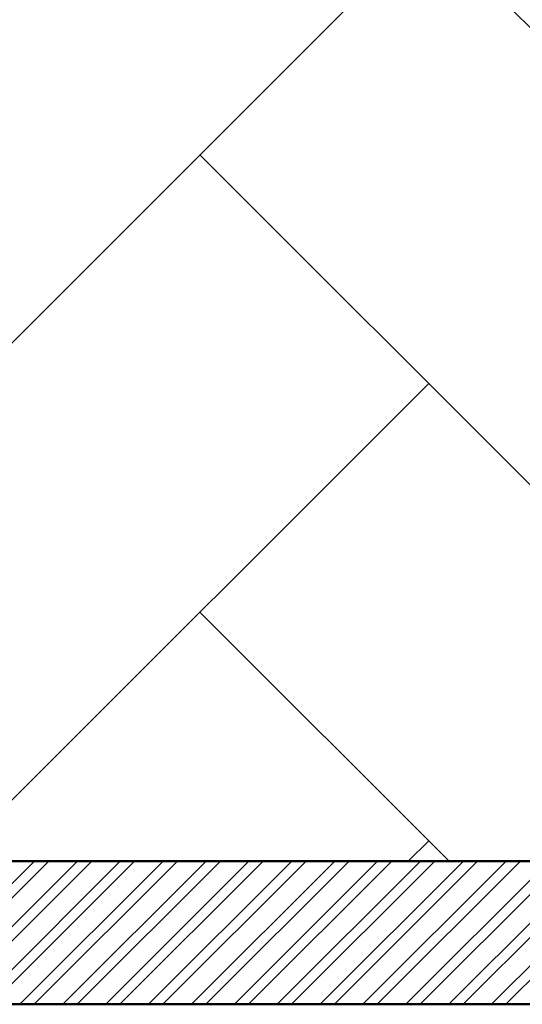
# Model space of a CAD drawing. Units: inches. Extents: x 3590 to 5167, y 65 to 1917.
# Tile 37 of 100: x 5003 to 5035, y 1326 to 1388. Entities that reach past the tile are written whole.
import ezdxf

# ---------------------------------------------------------------- set-up
doc = ezdxf.new("R2010")
doc.units = ezdxf.units.IN
for name, color, linetype, lineweight in [('A-FLOR-PATT', 8, 'Continuous', 13), ('A-WALL', 7, 'Continuous', 50), ('A-WALL-PATT', 251, 'Continuous', 13)]:
    doc.layers.add(name, color=color, linetype=linetype, lineweight=lineweight)

msp = doc.modelspace()

# ---------------------------------------------------------------- hatches: boundary and pattern name
at = {"layer": 'A-FLOR-PATT', "transparency": 33554687}
h = msp.add_hatch(dxfattribs=at)
h.set_pattern_fill('AR-HBONE', color=256, scale=0.2)
h.set_pattern_definition([(45, (-588.972, 0), (0, 28.73682), [60.96, -20.32]), (135, (-574.604, 14.368), (3e-15, 28.73682), [60.96, -20.32])])
h.paths.add_polyline_path([(5071.274, 1796.999), (4933.274, 1796.999), (4933.274, 1753.999), (4962.774, 1753.999, -0.414214), (4928.774, 1719.999), (4933.274, 1718.999), (4933.274, 1334.999), (5071.274, 1334.999)])
h.paths.add_polyline_path([(4951.78, 1521.077), (4951.715, 1521.04), (4951.563, 1520.895)], flags=16)
h.paths.add_polyline_path([(4952.267, 1521.376), (4952.198, 1521.371), (4952.198, 1521.356)], flags=0)
h.paths.add_polyline_path([(4967.051, 1529.728), (4965.231, 1528.694), (4963.411, 1527.714), (4961.756, 1526.851), (4963.589, 1527.449), (4964.036, 1527.478), (4962.975, 1527.249), (4961.76, 1526.852), (4959.792, 1525.834), (4958.005, 1524.895), (4956.24, 1523.93), (4954.504, 1522.919), (4954.129, 1522.682), (4953.361, 1521.997), (4953.366, 1521.998), (4953.605, 1522.064), (4955.106, 1522.761), (4956.921, 1523.434), (4958.678, 1523.915), (4960.358, 1524.2), (4961.945, 1524.286), (4964.171, 1524.108), (4965.958, 1523.309), (4963.863, 1522.976), (4965.187, 1522.499), (4963.366, 1522.497), (4961.545, 1522.487), (4959.764, 1522.461), (4958.304, 1522.419), (4957.974, 1522.388), (4956.307, 1522.232), (4954.718, 1522.071), (4953.251, 1521.899), (4953.525, 1521.623), (4954.331, 1521.379), (4956.243, 1521.23), (4958.039, 1520.93), (4959.684, 1520.483), (4961.16, 1519.896), (4963.107, 1518.8), (4964.393, 1517.325), (4962.973, 1517.726), (4964.558, 1516.661), (4965.407, 1515.708), (4963.507, 1516.322), (4961.68, 1517.005), (4959.935, 1517.745), (4958.282, 1518.528), (4956.732, 1519.343), (4955.295, 1520.175), (4954.672, 1520.572), (4954.513, 1520.627), (4955.658, 1519.318), (4956.703, 1517.982), (4957.644, 1516.647), (4958.485, 1515.334), (4959.55, 1513.524), (4960.438, 1511.769), (4958.841, 1513.62), (4957.452, 1515.325), (4955.819, 1517.459), (4956.665, 1515.448), (4957.111, 1513.923), (4957.447, 1511.714), (4957.076, 1509.793), (4956.538, 1511.11), (4955.992, 1512.569), (4955.444, 1514.125), (4954.898, 1515.735), (4954.357, 1517.356), (4953.824, 1518.943), (4953.305, 1520.452), (4953.065, 1521.116), (4952.971, 1521.146), (4952.949, 1521.086), (4952.73, 1520.199), (4953.37, 1518.024), (4953.757, 1516.373), (4954.051, 1514.765), (4954.264, 1513.221), (4954.471, 1511.131), (4954.497, 1510.402), (4954.409, 1511.76), (4954.264, 1513.221), (4954.051, 1514.765), (4953.757, 1516.373), (4953.37, 1518.024), (4952.877, 1519.698), (4952.716, 1520.141), (4952.533, 1519.059), (4952.374, 1517.789), (4952.219, 1516.312), (4952.046, 1514.6), (4951.833, 1512.626), (4951.557, 1510.363), (4951.203, 1512.168), (4950.852, 1514.339), (4950.985, 1516.376), (4951.66, 1518.286), (4952.593, 1520.481), (4952.357, 1521.13), (4951.855, 1520.328), (4950.839, 1518.908), (4949.777, 1517.587), (4948.916, 1516.617), (4948.111, 1515.256), (4947.089, 1513.554), (4945.889, 1511.615), (4946.326, 1513.402), (4946.562, 1514.249), (4945.528, 1513.327), (4944.581, 1512.531), (4946.018, 1514.508), (4947.204, 1516.048), (4947.893, 1517.313), (4949.307, 1518.764), (4950.414, 1519.767), (4950.451, 1519.806), (4952.267, 1521.376), (4951.645, 1521.493), (4950.404, 1521.18), (4948.044, 1520.359), (4946.119, 1519.452), (4944.572, 1518.475), (4943.35, 1517.443), (4941.997, 1515.92), (4941.661, 1515.275), (4942.813, 1516.99), (4944.572, 1518.475), (4946.119, 1519.452), (4948.044, 1520.359), (4950.404, 1521.18), (4951.645, 1521.493), (4949.647, 1521.868), (4948.6, 1521.756), (4947.126, 1521.57), (4945.42, 1521.348), (4943.45, 1521.105), (4941.183, 1520.856), (4942.86, 1521.613), (4943.873, 1522.03), (4942.952, 1521.909), (4941.41, 1521.485), (4939.543, 1520.67), (4938.968, 1520.226), (4940.733, 1521.299), (4942.952, 1521.909), (4943.702, 1522.008), (4945.894, 1522.7), (4947.565, 1522.714), (4948.921, 1522.566), (4951.131, 1522.183), (4950.971, 1522.297), (4948.129, 1523.006), (4946.035, 1523.707), (4944.232, 1524.521), (4942.707, 1525.461), (4941.444, 1526.537), (4940.43, 1527.761), (4939.649, 1529.143), (4941.421, 1528.122), (4943.147, 1527.132), (4944.841, 1526.175), (4946.514, 1525.25), (4948.179, 1524.359), (4948.365, 1524.263), (4946.475, 1526.045), (4945.181, 1527.54), (4944.19, 1529.033), (4943.496, 1530.54), (4943.278, 1531.36), (4942.498, 1531.919), (4943.114, 1531.762), (4942.959, 1533.659), (4944.14, 1531.989), (4944.612, 1531.323), (4946.202, 1530.463), (4947.486, 1529.509), (4948.79, 1528.226), (4950.368, 1526.237), (4949.485, 1528.155), (4948.851, 1530.123), (4948.491, 1532.041), (4948.381, 1533.918), (4948.501, 1535.76), (4948.827, 1537.573), (4949.418, 1535.565), (4949.957, 1533.569), (4950.464, 1531.586), (4950.961, 1529.617), (4951.391, 1527.954), (4951.724, 1530.687), (4952.201, 1532.58), (4952.889, 1534.33), (4953.77, 1535.951), (4954.827, 1537.46), (4954.521, 1535.39), (4954.273, 1533.937), (4955.58, 1535.663), (4956.748, 1536.739), (4956.159, 1534.78), (4955.589, 1532.873), (4955.043, 1531.006), (4954.525, 1529.166), (4954.038, 1527.341), (4953.638, 1525.733), (4953.611, 1525.586), (4953.398, 1524.166), (4953.382, 1524.009), (4954.07, 1525.476), (4954.912, 1527.022), (4956.136, 1528.894), (4957.847, 1530.577), (4959.376, 1531.54), (4958.256, 1530.104), (4957.143, 1528.663), (4956.066, 1527.243), (4955.056, 1525.871), (4954.141, 1524.571), (4953.352, 1523.372), (4953.311, 1523.303), (4953.273, 1522.925), (4953.261, 1522.382), (4954.103, 1523.373), (4954.63, 1524.284), (4955.961, 1526.358), (4957.23, 1528.13), (4958.421, 1529.609), (4960.037, 1531.368), (4961.374, 1532.375), (4962.101, 1532.77), (4961.07, 1531.061), (4959.987, 1529.438), (4958.869, 1527.908), (4958.15, 1527.007), (4959.803, 1528.003), (4961.589, 1528.793), (4963.391, 1529.328), (4965.211, 1529.632)], flags=16)
h.paths.add_polyline_path([(4962.944, 1523.182), (4961.107, 1523.422), (4960.392, 1523.362), (4962.35, 1523.331)], flags=0)
h.paths.add_polyline_path([(5049.541, 1584.551), (5049.476, 1584.515), (5049.325, 1584.37)], flags=16)
h.paths.add_polyline_path([(5050.028, 1584.851), (5049.959, 1584.845), (5049.959, 1584.83)], flags=0)
h.paths.add_polyline_path([(5042.333, 1581.949), (5043.88, 1582.926), (5045.806, 1583.833), (5048.165, 1584.654), (5049.406, 1584.967), (5047.408, 1585.342), (5046.361, 1585.231), (5044.888, 1585.044), (5043.181, 1584.822), (5041.211, 1584.579), (5038.944, 1584.33), (5040.622, 1585.087), (5041.634, 1585.504), (5040.713, 1585.383), (5039.171, 1584.959), (5037.304, 1584.144), (5036.729, 1583.7), (5038.494, 1584.773), (5040.713, 1585.383), (5041.463, 1585.482), (5043.655, 1586.174), (5045.326, 1586.188), (5046.682, 1586.04), (5048.893, 1585.657), (5048.732, 1585.771), (5045.891, 1586.48), (5043.796, 1587.181), (5041.994, 1587.996), (5040.468, 1588.935), (5039.205, 1590.011), (5038.191, 1591.235), (5037.41, 1592.617), (5039.182, 1591.596), (5040.909, 1590.607), (5042.602, 1589.649), (5044.275, 1588.724), (5045.94, 1587.833), (5046.126, 1587.738), (5044.237, 1589.519), (5042.942, 1591.015), (5041.952, 1592.508), (5041.257, 1594.014), (5041.039, 1594.834), (5040.26, 1595.393), (5040.875, 1595.237), (5040.721, 1597.133), (5041.901, 1595.463), (5042.373, 1594.798), (5043.963, 1593.938), (5045.247, 1592.983), (5046.552, 1591.701), (5048.129, 1589.712), (5047.247, 1591.63), (5046.613, 1593.597), (5046.252, 1595.515), (5046.142, 1597.392), (5046.262, 1599.234), (5046.588, 1601.047), (5047.179, 1599.039), (5047.718, 1597.043), (5048.225, 1595.06), (5048.722, 1593.091), (5049.152, 1591.429), (5049.485, 1594.161), (5049.962, 1596.054), (5050.65, 1597.804), (5051.532, 1599.425), (5052.589, 1600.934), (5052.283, 1598.864), (5052.034, 1597.411), (5053.341, 1599.137), (5054.509, 1600.213), (5053.92, 1598.254), (5053.35, 1596.348), (5052.805, 1594.48), (5052.286, 1592.64), (5051.799, 1590.815), (5051.4, 1589.207), (5051.373, 1589.06), (5051.159, 1587.64), (5051.143, 1587.483), (5051.831, 1588.95), (5052.673, 1590.496), (5053.898, 1592.368), (5055.608, 1594.051), (5057.137, 1595.014), (5056.017, 1593.578), (5054.904, 1592.137), (5053.828, 1590.717), (5052.817, 1589.345), (5051.902, 1588.046), (5051.113, 1586.846), (5051.072, 1586.777), (5051.034, 1586.399), (5051.022, 1585.856), (5051.864, 1586.847), (5052.391, 1587.758), (5053.723, 1589.832), (5054.991, 1591.604), (5056.182, 1593.083), (5057.798, 1594.842), (5059.135, 1595.849), (5059.863, 1596.244), (5058.831, 1594.535), (5057.749, 1592.912), (5056.63, 1591.382), (5055.912, 1590.482), (5057.564, 1591.477), (5059.35, 1592.267), (5061.152, 1592.802), (5062.972, 1593.106), (5064.812, 1593.203), (5062.992, 1592.169), (5061.172, 1591.188), (5059.518, 1590.325), (5061.35, 1590.924), (5061.797, 1590.952), (5060.737, 1590.723), (5059.521, 1590.326), (5057.553, 1589.308), (5055.766, 1588.369), (5054.002, 1587.404), (5052.265, 1586.393), (5051.891, 1586.156), (5051.122, 1585.471), (5051.127, 1585.472), (5051.366, 1585.538), (5052.867, 1586.235), (5054.682, 1586.908), (5056.439, 1587.389), (5058.12, 1587.675), (5059.706, 1587.76), (5061.933, 1587.583), (5063.719, 1586.783), (5061.624, 1586.45), (5062.949, 1585.973), (5061.127, 1585.971), (5059.307, 1585.961), (5057.525, 1585.935), (5056.065, 1585.893), (5055.735, 1585.862), (5054.068, 1585.707), (5052.479, 1585.546), (5051.012, 1585.373), (5051.286, 1585.097), (5052.092, 1584.853), (5054.004, 1584.704), (5055.8, 1584.404), (5057.446, 1583.958), (5058.921, 1583.37), (5060.868, 1582.274), (5062.154, 1580.799), (5060.734, 1581.2), (5062.32, 1580.135), (5063.168, 1579.182), (5061.269, 1579.796), (5059.441, 1580.479), (5057.696, 1581.219), (5056.043, 1582.003), (5054.493, 1582.817), (5053.057, 1583.649), (5052.433, 1584.047), (5052.274, 1584.101), (5053.42, 1582.793), (5054.464, 1581.457), (5055.405, 1580.121), (5056.247, 1578.809), (5057.311, 1576.998), (5058.199, 1575.244), (5056.602, 1577.094), (5055.213, 1578.799), (5053.58, 1580.933), (5054.427, 1578.922), (5054.872, 1577.397), (5055.208, 1575.189), (5054.838, 1573.267), (5054.299, 1574.584), (5053.754, 1576.043), (5053.206, 1577.599), (5052.659, 1579.209), (5052.118, 1580.83), (5051.585, 1582.417), (5051.066, 1583.927), (5050.826, 1584.59), (5050.733, 1584.62), (5050.711, 1584.561), (5050.491, 1583.673), (5051.131, 1581.498), (5051.518, 1579.847), (5051.813, 1578.24), (5052.026, 1576.695), (5052.233, 1574.605), (5052.258, 1573.876), (5052.17, 1575.234), (5052.026, 1576.695), (5051.813, 1578.24), (5051.518, 1579.847), (5051.131, 1581.498), (5050.638, 1583.172), (5050.477, 1583.615), (5050.294, 1582.533), (5050.136, 1581.263), (5049.981, 1579.786), (5049.807, 1578.074), (5049.594, 1576.1), (5049.318, 1573.837), (5048.965, 1575.642), (5048.613, 1577.813), (5048.747, 1579.85), (5049.421, 1581.76), (5050.354, 1583.955), (5050.118, 1584.604), (5049.616, 1583.802), (5048.6, 1582.382), (5047.538, 1581.061), (5046.677, 1580.091), (5045.872, 1578.73), (5044.85, 1577.028), (5043.651, 1575.089), (5044.087, 1576.877), (5044.324, 1577.723), (5043.289, 1576.801), (5042.342, 1576.005), (5043.779, 1577.982), (5044.966, 1579.522), (5045.655, 1580.787), (5047.068, 1582.239), (5048.175, 1583.241), (5048.213, 1583.28), (5050.028, 1584.851), (5049.406, 1584.967), (5048.165, 1584.654), (5045.806, 1583.833), (5043.88, 1582.926), (5042.333, 1581.949), (5041.111, 1580.917), (5039.758, 1579.394), (5039.423, 1578.749), (5040.575, 1580.464)], flags=16)
h.paths.add_polyline_path([(4954.799, 1533.12), (4954.262, 1532.079), (4953.831, 1530.935), (4953.505, 1529.636), (4953.283, 1528.133), (4953.167, 1526.376), (4953.156, 1524.315), (4953.277, 1521.236), (4952.802, 1521.842), (4951.557, 1521.998), (4950.976, 1521.961), (4952.661, 1521.941), (4952.802, 1521.842), (4953.152, 1523.593), (4953.167, 1526.376), (4953.283, 1528.133), (4953.609, 1530.346), (4954.456, 1532.592)], flags=0)
h.paths.add_polyline_path([(5050.563, 1585.316), (5049.318, 1585.472), (5048.737, 1585.435), (5050.422, 1585.415), (5050.563, 1585.316), (5050.914, 1587.067), (5050.928, 1589.851), (5051.045, 1591.607), (5051.371, 1593.82), (5052.217, 1596.066), (5052.56, 1596.594), (5052.024, 1595.554), (5051.592, 1594.409), (5051.266, 1593.11), (5051.045, 1591.607), (5050.928, 1589.851), (5050.918, 1587.789), (5051.038, 1584.71)], flags=0)
h.paths.add_polyline_path([(5058.153, 1586.836), (5060.111, 1586.805), (5060.705, 1586.656), (5058.868, 1586.896)], flags=0)
h.paths.add_polyline_path([(5049.541, 1430.936), (5049.476, 1430.9), (5049.325, 1430.755)], flags=16)
h.paths.add_polyline_path([(5050.028, 1431.236), (5049.959, 1431.231), (5049.959, 1431.215)], flags=0)
h.paths.add_polyline_path([(5046.588, 1447.432), (5047.179, 1445.425), (5047.718, 1443.429), (5048.225, 1441.446), (5048.722, 1439.476), (5049.152, 1437.814), (5049.485, 1440.546), (5049.962, 1442.439), (5050.65, 1444.189), (5051.532, 1445.811), (5052.589, 1447.319), (5052.283, 1445.249), (5052.034, 1443.796), (5053.341, 1445.522), (5054.509, 1446.598), (5053.92, 1444.64), (5053.35, 1442.733), (5052.805, 1440.865), (5052.286, 1439.025), (5051.799, 1437.201), (5051.4, 1435.592), (5051.373, 1435.445), (5051.159, 1434.025), (5051.143, 1433.868), (5051.831, 1435.335), (5052.673, 1436.881), (5053.898, 1438.753), (5055.608, 1440.436), (5057.137, 1441.4), (5056.017, 1439.963), (5054.904, 1438.522), (5053.828, 1437.102), (5052.817, 1435.73), (5051.902, 1434.431), (5051.113, 1433.231), (5051.072, 1433.162), (5051.034, 1432.784), (5051.022, 1432.242), (5051.864, 1433.232), (5052.391, 1434.143), (5053.723, 1436.217), (5054.991, 1437.989), (5056.182, 1439.468), (5057.798, 1441.227), (5059.135, 1442.235), (5059.863, 1442.629), (5058.831, 1440.921), (5057.749, 1439.298), (5056.63, 1437.767), (5055.912, 1436.867), (5057.564, 1437.863), (5059.35, 1438.652), (5061.152, 1439.187), (5062.972, 1439.491), (5064.812, 1439.588), (5062.992, 1438.554), (5061.172, 1437.573), (5059.518, 1436.71), (5061.35, 1437.309), (5061.797, 1437.337), (5060.737, 1437.108), (5059.521, 1436.711), (5057.553, 1435.693), (5055.766, 1434.754), (5054.002, 1433.789), (5052.265, 1432.778), (5051.891, 1432.541), (5051.122, 1431.856), (5051.127, 1431.857), (5051.366, 1431.923), (5052.867, 1432.62), (5054.682, 1433.293), (5056.439, 1433.775), (5058.12, 1434.06), (5059.706, 1434.145), (5061.933, 1433.968), (5063.719, 1433.168), (5061.624, 1432.835), (5062.949, 1432.358), (5061.127, 1432.357), (5059.307, 1432.346), (5057.525, 1432.32), (5056.065, 1432.278), (5055.735, 1432.248), (5054.068, 1432.092), (5052.479, 1431.931), (5051.012, 1431.759), (5051.286, 1431.482), (5052.092, 1431.238), (5054.004, 1431.089), (5055.8, 1430.789), (5057.446, 1430.343), (5058.921, 1429.755), (5060.868, 1428.66), (5062.154, 1427.185), (5060.734, 1427.585), (5062.32, 1426.52), (5063.168, 1425.567), (5061.269, 1426.181), (5059.441, 1426.865), (5057.696, 1427.604), (5056.043, 1428.388), (5054.493, 1429.202), (5053.057, 1430.034), (5052.433, 1430.432), (5052.274, 1430.487), (5053.42, 1429.178), (5054.464, 1427.842), (5055.405, 1426.506), (5056.247, 1425.194), (5057.311, 1423.383), (5058.199, 1421.629), (5056.602, 1423.479), (5055.213, 1425.184), (5053.58, 1427.318), (5054.427, 1425.307), (5054.872, 1423.782), (5055.208, 1421.574), (5054.838, 1419.652), (5054.299, 1420.97), (5053.754, 1422.428), (5053.206, 1423.984), (5052.659, 1425.595), (5052.118, 1427.215), (5051.585, 1428.802), (5051.066, 1430.312), (5050.826, 1430.975), (5050.733, 1431.005), (5050.711, 1430.946), (5050.491, 1430.058), (5051.131, 1427.883), (5051.518, 1426.232), (5051.813, 1424.625), (5052.026, 1423.081), (5052.233, 1420.991), (5052.258, 1420.261), (5052.17, 1421.619), (5052.026, 1423.081), (5051.813, 1424.625), (5051.518, 1426.232), (5051.131, 1427.883), (5050.638, 1429.558), (5050.477, 1430.001), (5050.294, 1428.918), (5050.136, 1427.648), (5049.981, 1426.171), (5049.807, 1424.459), (5049.594, 1422.485), (5049.318, 1420.222), (5048.965, 1422.028), (5048.613, 1424.199), (5048.747, 1426.235), (5049.421, 1428.146), (5050.354, 1430.34), (5050.118, 1430.989), (5049.616, 1430.187), (5048.6, 1428.768), (5047.538, 1427.446), (5046.677, 1426.477), (5045.872, 1425.116), (5044.85, 1423.413), (5043.651, 1421.474), (5044.087, 1423.262), (5044.324, 1424.109), (5043.289, 1423.186), (5042.342, 1422.391), (5043.779, 1424.368), (5044.966, 1425.907), (5045.655, 1427.173), (5047.068, 1428.624), (5048.175, 1429.627), (5048.213, 1429.666), (5050.028, 1431.236), (5049.406, 1431.353), (5048.165, 1431.039), (5045.806, 1430.218), (5043.88, 1429.311), (5042.333, 1428.334), (5041.111, 1427.302), (5039.758, 1425.779), (5039.423, 1425.134), (5040.575, 1426.849), (5042.333, 1428.334), (5043.88, 1429.311), (5045.806, 1430.218), (5048.165, 1431.039), (5049.406, 1431.353), (5047.408, 1431.727), (5046.361, 1431.616), (5044.888, 1431.429), (5043.181, 1431.207), (5041.211, 1430.964), (5038.944, 1430.715), (5040.622, 1431.472), (5041.634, 1431.89), (5040.713, 1431.769), (5039.171, 1431.345), (5037.304, 1430.53), (5036.729, 1430.085), (5038.494, 1431.158), (5040.713, 1431.769), (5041.463, 1431.867), (5043.655, 1432.559), (5045.326, 1432.573), (5046.682, 1432.425), (5048.893, 1432.042), (5048.732, 1432.156), (5045.891, 1432.865), (5043.796, 1433.566), (5041.994, 1434.381), (5040.468, 1435.321), (5039.205, 1436.396), (5038.191, 1437.62), (5037.41, 1439.002), (5039.182, 1437.982), (5040.909, 1436.992), (5042.602, 1436.034), (5044.275, 1435.109), (5045.94, 1434.218), (5046.126, 1434.123), (5044.237, 1435.904), (5042.942, 1437.4), (5041.952, 1438.893), (5041.257, 1440.399), (5041.039, 1441.219), (5040.26, 1441.778), (5040.875, 1441.622), (5040.721, 1443.518), (5041.901, 1441.848), (5042.373, 1441.183), (5043.963, 1440.323), (5045.247, 1439.369), (5046.552, 1438.086), (5048.129, 1436.097), (5047.247, 1438.015), (5046.613, 1439.982), (5046.252, 1441.901), (5046.142, 1443.778), (5046.262, 1445.619)], flags=16)
h.paths.add_polyline_path([(5052.382, 1444.255), (5051.623, 1442.78), (5052.024, 1441.939), (5052.56, 1442.98)], flags=0)
h.paths.add_polyline_path([(5050.563, 1431.701), (5049.318, 1431.857), (5048.737, 1431.821), (5050.422, 1431.8)], flags=0)
h.paths.add_polyline_path([(5058.153, 1433.221), (5060.111, 1433.19), (5060.705, 1433.041), (5058.868, 1433.281)], flags=0)
h.paths.add_polyline_path([(5049.541, 1352.285), (5049.476, 1352.249), (5049.325, 1352.104)], flags=16)
h.paths.add_polyline_path([(5050.028, 1352.585), (5049.959, 1352.58), (5049.959, 1352.564)], flags=0)
h.paths.add_polyline_path([(5046.588, 1368.781), (5047.179, 1366.774), (5047.718, 1364.778), (5048.225, 1362.795), (5048.722, 1360.825), (5049.152, 1359.163), (5049.485, 1361.896), (5049.962, 1363.789), (5050.65, 1365.538), (5051.532, 1367.16), (5052.589, 1368.669), (5052.283, 1366.598), (5052.034, 1365.145), (5053.341, 1366.871), (5054.509, 1367.947), (5053.92, 1365.989), (5053.35, 1364.082), (5052.805, 1362.214), (5052.286, 1360.374), (5051.799, 1358.55), (5051.4, 1356.942), (5051.373, 1356.794), (5051.159, 1355.374), (5051.143, 1355.218), (5051.831, 1356.684), (5052.673, 1358.23), (5053.898, 1360.102), (5055.608, 1361.786), (5057.137, 1362.749), (5056.017, 1361.313), (5054.904, 1359.872), (5053.828, 1358.452), (5052.817, 1357.079), (5051.902, 1355.78), (5051.113, 1354.581), (5051.072, 1354.512), (5051.034, 1354.133), (5051.022, 1353.591), (5051.864, 1354.581), (5052.391, 1355.492), (5053.723, 1357.566), (5054.991, 1359.338), (5056.182, 1360.817), (5057.798, 1362.577), (5059.135, 1363.584), (5059.863, 1363.979), (5058.831, 1362.27), (5057.749, 1360.647), (5056.63, 1359.117), (5055.912, 1358.216), (5057.564, 1359.212), (5059.35, 1360.001), (5061.152, 1360.536), (5062.972, 1360.841), (5064.812, 1360.937), (5062.992, 1359.903), (5061.172, 1358.923), (5059.518, 1358.059), (5061.35, 1358.658), (5061.797, 1358.687), (5060.737, 1358.458), (5059.521, 1358.061), (5057.553, 1357.043), (5055.766, 1356.103), (5054.002, 1355.138), (5052.265, 1354.127), (5051.891, 1353.89), (5051.122, 1353.206), (5051.127, 1353.206), (5051.366, 1353.272), (5052.867, 1353.969), (5054.682, 1354.643), (5056.439, 1355.124), (5058.12, 1355.409), (5059.706, 1355.495), (5061.933, 1355.317), (5063.719, 1354.518), (5061.624, 1354.184), (5062.949, 1353.708), (5061.127, 1353.706), (5059.307, 1353.695), (5057.525, 1353.669), (5056.065, 1353.627), (5055.735, 1353.597), (5054.068, 1353.441), (5052.479, 1353.28), (5051.012, 1353.108), (5051.286, 1352.831), (5052.092, 1352.587), (5054.004, 1352.439), (5055.8, 1352.138), (5057.446, 1351.692), (5058.921, 1351.104), (5060.868, 1350.009), (5062.154, 1348.534), (5060.734, 1348.935), (5062.32, 1347.869), (5063.168, 1346.916), (5061.269, 1347.53), (5059.441, 1348.214), (5057.696, 1348.954), (5056.043, 1349.737), (5054.493, 1350.551), (5053.057, 1351.383), (5052.433, 1351.781), (5052.274, 1351.836), (5053.42, 1350.527), (5054.464, 1349.191), (5055.405, 1347.855), (5056.247, 1346.543), (5057.311, 1344.733), (5058.199, 1342.978), (5056.602, 1344.828), (5055.213, 1346.534), (5053.58, 1348.667), (5054.427, 1346.656), (5054.872, 1345.132), (5055.208, 1342.923), (5054.838, 1341.002), (5054.299, 1342.319), (5053.754, 1343.778), (5053.206, 1345.334), (5052.659, 1346.944), (5052.118, 1348.564), (5051.585, 1350.151), (5051.066, 1351.661), (5050.826, 1352.324), (5050.733, 1352.355), (5050.711, 1352.295), (5050.491, 1351.408), (5051.131, 1349.232), (5051.518, 1347.581), (5051.813, 1345.974), (5052.026, 1344.43), (5052.233, 1342.34), (5052.258, 1341.61), (5052.17, 1342.969), (5052.026, 1344.43), (5051.813, 1345.974), (5051.518, 1347.581), (5051.131, 1349.232), (5050.638, 1350.907), (5050.477, 1351.35), (5050.294, 1350.267), (5050.136, 1348.997), (5049.981, 1347.52), (5049.807, 1345.809), (5049.594, 1343.835), (5049.318, 1341.571), (5048.965, 1343.377), (5048.613, 1345.548), (5048.747, 1347.585), (5049.421, 1349.495), (5050.354, 1351.689), (5050.118, 1352.339), (5049.616, 1351.536), (5048.6, 1350.117), (5047.538, 1348.795), (5046.677, 1347.826), (5045.872, 1346.465), (5044.85, 1344.763), (5043.651, 1342.824), (5044.087, 1344.611), (5044.324, 1345.458), (5043.289, 1344.535), (5042.342, 1343.74), (5043.779, 1345.717), (5044.966, 1347.256), (5045.655, 1348.522), (5047.068, 1349.973), (5048.175, 1350.976), (5048.213, 1351.015), (5050.028, 1352.585), (5049.406, 1352.702), (5048.165, 1352.388), (5045.806, 1351.567), (5043.88, 1350.661), (5042.333, 1349.683), (5041.111, 1348.651), (5039.758, 1347.128), (5039.423, 1346.483), (5040.575, 1348.198), (5042.333, 1349.683), (5043.88, 1350.661), (5045.806, 1351.567), (5048.165, 1352.388), (5049.406, 1352.702), (5047.408, 1353.076), (5046.361, 1352.965), (5044.888, 1352.779), (5043.181, 1352.556), (5041.211, 1352.313), (5038.944, 1352.065), (5040.622, 1352.821), (5041.634, 1353.239), (5040.713, 1353.118), (5039.171, 1352.694), (5037.304, 1351.879), (5036.729, 1351.434), (5038.494, 1352.508), (5040.713, 1353.118), (5041.463, 1353.216), (5043.655, 1353.909), (5045.326, 1353.923), (5046.682, 1353.774), (5048.893, 1353.391), (5048.732, 1353.506), (5045.891, 1354.214), (5043.796, 1354.915), (5041.994, 1355.73), (5040.468, 1356.67), (5039.205, 1357.746), (5038.191, 1358.969), (5037.41, 1360.352), (5039.182, 1359.331), (5040.909, 1358.341), (5042.602, 1357.383), (5044.275, 1356.458), (5045.94, 1355.567), (5046.126, 1355.472), (5044.237, 1357.253), (5042.942, 1358.749), (5041.952, 1360.242), (5041.257, 1361.748), (5041.039, 1362.568), (5040.26, 1363.128), (5040.875, 1362.971), (5040.721, 1364.867), (5041.901, 1363.197), (5042.373, 1362.532), (5043.963, 1361.672), (5045.247, 1360.718), (5046.552, 1359.435), (5048.129, 1357.446), (5047.247, 1359.364), (5046.613, 1361.331), (5046.252, 1363.25), (5046.142, 1365.127), (5046.262, 1366.969)], flags=16)
h.paths.add_polyline_path([(5052.382, 1365.604), (5051.623, 1364.129), (5052.024, 1363.288), (5052.56, 1364.329)], flags=0)
h.paths.add_polyline_path([(4951.78, 1698.041), (4951.715, 1698.005), (4951.563, 1697.859)], flags=16)
h.paths.add_polyline_path([(4952.267, 1698.341), (4952.198, 1698.335), (4952.198, 1698.32)], flags=0)
h.paths.add_polyline_path([(4957.076, 1686.757), (4956.538, 1688.074), (4955.992, 1689.533), (4955.444, 1691.089), (4954.898, 1692.699), (4954.357, 1694.32), (4953.824, 1695.907), (4953.305, 1697.417), (4953.065, 1698.08), (4952.971, 1698.11), (4952.949, 1698.051), (4952.73, 1697.163), (4953.37, 1694.988), (4953.757, 1693.337), (4954.051, 1691.729), (4954.264, 1690.185), (4954.471, 1688.095), (4954.497, 1687.366), (4954.409, 1688.724), (4954.264, 1690.185), (4954.051, 1691.729), (4953.757, 1693.337), (4953.37, 1694.988), (4952.877, 1696.662), (4952.716, 1697.105), (4952.533, 1696.023), (4952.374, 1694.753), (4952.219, 1693.276), (4952.046, 1691.564), (4951.833, 1689.59), (4951.557, 1687.327), (4951.203, 1689.132), (4950.852, 1691.303), (4950.985, 1693.34), (4951.66, 1695.25), (4952.593, 1697.445), (4952.357, 1698.094), (4951.855, 1697.292), (4950.839, 1695.872), (4949.777, 1694.551), (4948.916, 1693.581), (4948.111, 1692.22), (4947.089, 1690.518), (4945.889, 1688.579), (4946.326, 1690.366), (4946.562, 1691.213), (4945.528, 1690.291), (4944.581, 1689.495), (4946.018, 1691.472), (4947.204, 1693.012), (4947.893, 1694.277), (4949.307, 1695.729), (4950.414, 1696.731), (4950.451, 1696.77), (4952.267, 1698.341), (4951.645, 1698.457), (4950.404, 1698.144), (4948.044, 1697.323), (4946.119, 1696.416), (4944.572, 1695.439), (4943.35, 1694.407), (4941.997, 1692.884), (4941.661, 1692.239), (4942.813, 1693.954), (4944.572, 1695.439), (4946.119, 1696.416), (4948.044, 1697.323), (4950.404, 1698.144), (4951.645, 1698.457), (4949.647, 1698.832), (4948.6, 1698.72), (4947.126, 1698.534), (4945.42, 1698.312), (4943.45, 1698.069), (4941.183, 1697.82), (4942.86, 1698.577), (4943.873, 1698.994), (4942.952, 1698.873), (4941.41, 1698.449), (4939.543, 1697.634), (4938.968, 1697.19), (4940.733, 1698.263), (4942.952, 1698.873), (4943.702, 1698.972), (4945.894, 1699.664), (4947.565, 1699.678), (4948.921, 1699.53), (4951.131, 1699.147), (4950.971, 1699.261), (4948.129, 1699.97), (4946.035, 1700.671), (4944.232, 1701.486), (4942.707, 1702.425), (4941.444, 1703.501), (4940.43, 1704.725), (4939.649, 1706.107), (4941.421, 1705.086), (4943.147, 1704.097), (4944.841, 1703.139), (4946.514, 1702.214), (4948.179, 1701.323), (4948.365, 1701.227), (4946.475, 1703.009), (4945.181, 1704.505), (4944.19, 1705.997), (4943.496, 1707.504), (4943.278, 1708.324), (4942.498, 1708.883), (4943.114, 1708.727), (4942.959, 1710.623), (4944.14, 1708.953), (4944.612, 1708.287), (4946.202, 1707.428), (4947.486, 1706.473), (4948.79, 1705.191), (4950.368, 1703.202), (4949.485, 1705.12), (4948.851, 1707.087), (4948.491, 1709.005), (4948.381, 1710.882), (4948.501, 1712.724), (4948.827, 1714.537), (4949.418, 1712.529), (4949.957, 1710.533), (4950.464, 1708.55), (4950.961, 1706.581), (4951.391, 1704.919), (4951.724, 1707.651), (4952.201, 1709.544), (4952.889, 1711.294), (4953.77, 1712.915), (4954.827, 1714.424), (4954.521, 1712.354), (4954.273, 1710.901), (4955.58, 1712.627), (4956.748, 1713.703), (4956.159, 1711.744), (4955.589, 1709.837), (4955.043, 1707.97), (4954.525, 1706.13), (4954.038, 1704.305), (4953.638, 1702.697), (4953.611, 1702.55), (4953.398, 1701.13), (4953.382, 1700.973), (4954.07, 1702.44), (4954.912, 1703.986), (4956.136, 1705.858), (4957.847, 1707.541), (4959.376, 1708.504), (4958.256, 1707.068), (4957.143, 1705.627), (4956.066, 1704.207), (4955.056, 1702.835), (4954.141, 1701.536), (4953.352, 1700.336), (4953.311, 1700.267), (4953.273, 1699.889), (4953.261, 1699.346), (4954.103, 1700.337), (4954.63, 1701.248), (4955.961, 1703.322), (4957.23, 1705.094), (4958.421, 1706.573), (4960.037, 1708.332), (4961.374, 1709.339), (4962.101, 1709.734), (4961.07, 1708.025), (4959.987, 1706.402), (4958.869, 1704.872), (4958.15, 1703.972), (4959.803, 1704.967), (4961.589, 1705.757), (4963.391, 1706.292), (4965.211, 1706.596), (4967.051, 1706.692), (4965.231, 1705.659), (4963.411, 1704.678), (4961.756, 1703.815), (4963.589, 1704.413), (4964.036, 1704.442), (4962.975, 1704.213), (4961.76, 1703.816), (4959.792, 1702.798), (4958.005, 1701.859), (4956.24, 1700.894), (4954.504, 1699.883), (4954.129, 1699.646), (4953.361, 1698.961), (4953.366, 1698.962), (4953.605, 1699.028), (4955.106, 1699.725), (4956.921, 1700.398), (4958.678, 1700.879), (4960.358, 1701.164), (4961.945, 1701.25), (4964.171, 1701.073), (4965.958, 1700.273), (4963.863, 1699.94), (4965.187, 1699.463), (4963.366, 1699.461), (4961.545, 1699.451), (4959.764, 1699.425), (4958.304, 1699.383), (4957.974, 1699.352), (4956.307, 1699.197), (4954.718, 1699.036), (4953.251, 1698.863), (4953.525, 1698.587), (4954.331, 1698.343), (4956.243, 1698.194), (4958.039, 1697.894), (4959.684, 1697.447), (4961.16, 1696.86), (4963.107, 1695.764), (4964.393, 1694.289), (4962.973, 1694.69), (4964.558, 1693.625), (4965.407, 1692.672), (4963.507, 1693.286), (4961.68, 1693.969), (4959.935, 1694.709), (4958.282, 1695.492), (4956.732, 1696.307), (4955.295, 1697.139), (4954.672, 1697.536), (4954.513, 1697.591), (4955.658, 1696.282), (4956.703, 1694.946), (4957.644, 1693.611), (4958.485, 1692.298), (4959.55, 1690.488), (4960.438, 1688.733), (4958.841, 1690.584), (4957.452, 1692.289), (4955.819, 1694.423), (4956.665, 1692.412), (4957.111, 1690.887), (4957.447, 1688.678)], flags=16)
h.paths.add_polyline_path([(5050.563, 1353.05), (5049.318, 1353.207), (5048.737, 1353.17), (5050.422, 1353.15)], flags=0)
h.paths.add_polyline_path([(4951.78, 1351.486), (4951.715, 1351.45), (4951.563, 1351.305)], flags=16)
h.paths.add_polyline_path([(4952.267, 1351.786), (4952.198, 1351.78), (4952.198, 1351.765)], flags=0)
h.paths.add_polyline_path([(4954.827, 1367.869), (4954.521, 1365.799), (4954.273, 1364.346), (4955.58, 1366.072), (4956.748, 1367.148), (4956.159, 1365.19), (4955.589, 1363.283), (4955.043, 1361.415), (4954.525, 1359.575), (4954.038, 1357.751), (4953.638, 1356.142), (4953.611, 1355.995), (4953.398, 1354.575), (4953.382, 1354.418), (4954.07, 1355.885), (4954.912, 1357.431), (4956.136, 1359.303), (4957.847, 1360.986), (4959.376, 1361.95), (4958.256, 1360.513), (4957.143, 1359.072), (4956.066, 1357.652), (4955.056, 1356.28), (4954.141, 1354.981), (4953.352, 1353.781), (4953.311, 1353.712), (4953.273, 1353.334), (4953.261, 1352.792), (4954.103, 1353.782), (4954.63, 1354.693), (4955.961, 1356.767), (4957.23, 1358.539), (4958.421, 1360.018), (4960.037, 1361.777), (4961.374, 1362.785), (4962.101, 1363.179), (4961.07, 1361.471), (4959.987, 1359.848), (4958.869, 1358.317), (4958.15, 1357.417), (4959.803, 1358.413), (4961.589, 1359.202), (4963.391, 1359.737), (4965.211, 1360.041), (4967.051, 1360.138), (4965.231, 1359.104), (4963.411, 1358.123), (4961.756, 1357.26), (4963.589, 1357.859), (4964.036, 1357.887), (4962.975, 1357.658), (4961.76, 1357.261), (4959.792, 1356.243), (4958.005, 1355.304), (4956.24, 1354.339), (4954.504, 1353.328), (4954.129, 1353.091), (4953.361, 1352.406), (4953.366, 1352.407), (4953.605, 1352.473), (4955.106, 1353.17), (4956.921, 1353.843), (4958.678, 1354.325), (4960.358, 1354.61), (4961.945, 1354.695), (4964.171, 1354.518), (4965.958, 1353.718), (4963.863, 1353.385), (4965.187, 1352.908), (4963.366, 1352.907), (4961.545, 1352.896), (4959.764, 1352.87), (4958.304, 1352.828), (4957.974, 1352.798), (4956.307, 1352.642), (4954.718, 1352.481), (4953.251, 1352.309), (4953.525, 1352.032), (4954.331, 1351.788), (4956.243, 1351.639), (4958.039, 1351.339), (4959.684, 1350.893), (4961.16, 1350.305), (4963.107, 1349.21), (4964.393, 1347.735), (4962.973, 1348.135), (4964.558, 1347.07), (4965.407, 1346.117), (4963.507, 1346.731), (4961.68, 1347.414), (4959.935, 1348.154), (4958.282, 1348.938), (4956.732, 1349.752), (4955.295, 1350.584), (4954.672, 1350.982), (4954.513, 1351.036), (4955.658, 1349.728), (4956.703, 1348.392), (4957.644, 1347.056), (4958.485, 1345.744), (4959.55, 1343.933), (4960.438, 1342.179), (4958.841, 1344.029), (4957.452, 1345.734), (4955.819, 1347.868), (4956.665, 1345.857), (4957.111, 1344.332), (4957.447, 1342.124), (4957.076, 1340.202), (4956.538, 1341.52), (4955.992, 1342.978), (4955.444, 1344.534), (4954.898, 1346.145), (4954.357, 1347.765), (4953.824, 1349.352), (4953.305, 1350.862), (4953.065, 1351.525), (4952.971, 1351.555), (4952.949, 1351.496), (4952.73, 1350.608), (4953.37, 1348.433), (4953.757, 1346.782), (4954.051, 1345.175), (4954.264, 1343.631), (4954.471, 1341.541), (4954.497, 1340.811), (4954.409, 1342.169), (4954.264, 1343.631), (4954.051, 1345.175), (4953.757, 1346.782), (4953.37, 1348.433), (4952.877, 1350.108), (4952.716, 1350.551), (4952.533, 1349.468), (4952.374, 1348.198), (4952.219, 1346.721), (4952.046, 1345.009), (4951.833, 1343.035), (4951.557, 1340.772), (4951.203, 1342.578), (4950.852, 1344.749), (4950.985, 1346.785), (4951.66, 1348.696), (4952.593, 1350.89), (4952.357, 1351.539), (4951.855, 1350.737), (4950.839, 1349.318), (4949.777, 1347.996), (4948.916, 1347.027), (4948.111, 1345.665), (4947.089, 1343.963), (4945.889, 1342.024), (4946.326, 1343.812), (4946.562, 1344.659), (4945.528, 1343.736), (4944.581, 1342.941), (4946.018, 1344.918), (4947.204, 1346.457), (4947.893, 1347.723), (4949.307, 1349.174), (4950.414, 1350.177), (4950.451, 1350.216), (4952.267, 1351.786), (4951.645, 1351.903), (4950.404, 1351.589), (4948.044, 1350.768), (4946.119, 1349.861), (4944.572, 1348.884), (4943.35, 1347.852), (4941.997, 1346.329), (4941.661, 1345.684), (4942.813, 1347.399), (4944.572, 1348.884), (4946.119, 1349.861), (4948.044, 1350.768), (4950.404, 1351.589), (4951.645, 1351.903), (4949.647, 1352.277), (4948.6, 1352.166), (4947.126, 1351.979), (4945.42, 1351.757), (4943.45, 1351.514), (4941.183, 1351.265), (4942.86, 1352.022), (4943.873, 1352.44), (4942.952, 1352.319), (4941.41, 1351.895), (4939.543, 1351.08), (4938.968, 1350.635), (4940.733, 1351.708), (4942.952, 1352.319), (4943.702, 1352.417), (4945.894, 1353.109), (4947.565, 1353.123), (4948.921, 1352.975), (4951.131, 1352.592), (4950.971, 1352.706), (4948.129, 1353.415), (4946.035, 1354.116), (4944.232, 1354.931), (4942.707, 1355.871), (4941.444, 1356.946), (4940.43, 1358.17), (4939.649, 1359.552), (4941.421, 1358.532), (4943.147, 1357.542), (4944.841, 1356.584), (4946.514, 1355.659), (4948.179, 1354.768), (4948.365, 1354.673), (4946.475, 1356.454), (4945.181, 1357.95), (4944.19, 1359.443), (4943.496, 1360.949), (4943.278, 1361.769), (4942.498, 1362.328), (4943.114, 1362.172), (4942.959, 1364.068), (4944.14, 1362.398), (4944.612, 1361.733), (4946.202, 1360.873), (4947.486, 1359.919), (4948.79, 1358.636), (4950.368, 1356.647), (4949.485, 1358.565), (4948.851, 1360.532), (4948.491, 1362.451), (4948.381, 1364.328), (4948.501, 1366.169), (4948.827, 1367.982), (4949.418, 1365.975), (4949.957, 1363.979), (4950.464, 1361.995), (4950.961, 1360.026), (4951.391, 1358.364), (4951.724, 1361.096), (4952.201, 1362.989), (4952.889, 1364.739), (4953.77, 1366.361)], flags=16)
h.paths.add_polyline_path([(4954.799, 1363.53), (4954.262, 1362.489), (4953.831, 1361.344), (4953.505, 1360.045), (4953.283, 1358.543), (4953.167, 1356.786), (4953.156, 1354.724), (4953.277, 1351.646), (4952.802, 1352.251), (4951.557, 1352.407), (4950.976, 1352.371), (4952.661, 1352.35), (4952.802, 1352.251), (4953.152, 1354.002), (4953.167, 1356.786), (4953.283, 1358.543), (4953.609, 1360.755), (4954.456, 1363.001)], flags=0)
h.paths.add_polyline_path([(4952.802, 1698.806), (4951.557, 1698.962), (4950.976, 1698.925), (4952.661, 1698.905), (4952.802, 1698.806), (4953.152, 1700.557), (4953.167, 1703.34), (4953.283, 1705.097), (4953.609, 1707.31), (4954.456, 1709.556), (4954.799, 1710.084), (4954.262, 1709.043), (4953.831, 1707.899), (4953.505, 1706.6), (4953.283, 1705.097), (4953.167, 1703.34), (4953.156, 1701.279), (4953.277, 1698.2)], flags=0)
h.paths.add_polyline_path([(4962.944, 1700.146), (4961.107, 1700.386), (4960.392, 1700.326), (4962.35, 1700.295)], flags=0)
h.paths.add_polyline_path([(5058.153, 1354.57), (5060.111, 1354.539), (5060.705, 1354.391), (5058.868, 1354.631)], flags=0)
h.paths.add_polyline_path([(4962.944, 1353.591), (4961.107, 1353.831), (4960.392, 1353.771), (4962.35, 1353.74)], flags=0)
h.paths.add_polyline_path([(5049.541, 1778.72), (5049.476, 1778.684), (5049.325, 1778.539)], flags=16)
h.paths.add_polyline_path([(5050.028, 1779.02), (5049.959, 1779.014), (5049.959, 1778.999)], flags=0)
h.paths.add_polyline_path([(5052.258, 1768.045), (5052.17, 1769.403), (5052.026, 1770.864), (5051.813, 1772.409), (5051.518, 1774.016), (5051.131, 1775.667), (5050.638, 1777.341), (5050.477, 1777.784), (5050.294, 1776.702), (5050.136, 1775.432), (5049.981, 1773.955), (5049.807, 1772.243), (5049.594, 1770.269), (5049.318, 1768.006), (5048.965, 1769.811), (5048.613, 1771.982), (5048.747, 1774.019), (5049.421, 1775.929), (5050.354, 1778.124), (5050.118, 1778.773), (5049.616, 1777.971), (5048.6, 1776.551), (5047.538, 1775.23), (5046.677, 1774.26), (5045.872, 1772.899), (5044.85, 1771.197), (5043.651, 1769.258), (5044.087, 1771.046), (5044.324, 1771.892), (5043.289, 1770.97), (5042.342, 1770.174), (5043.779, 1772.151), (5044.966, 1773.691), (5045.655, 1774.956), (5047.068, 1776.408), (5048.175, 1777.41), (5048.213, 1777.449), (5050.028, 1779.02), (5049.406, 1779.136), (5048.165, 1778.823), (5045.806, 1778.002), (5043.88, 1777.095), (5042.333, 1776.118), (5041.111, 1775.086), (5039.758, 1773.563), (5039.423, 1772.918), (5040.575, 1774.633), (5042.333, 1776.118), (5043.88, 1777.095), (5045.806, 1778.002), (5048.165, 1778.823), (5049.406, 1779.136), (5047.408, 1779.511), (5046.361, 1779.4), (5044.888, 1779.213), (5043.181, 1778.991), (5041.211, 1778.748), (5038.944, 1778.499), (5040.622, 1779.256), (5041.634, 1779.673), (5040.713, 1779.552), (5039.171, 1779.128), (5037.304, 1778.313), (5036.729, 1777.869), (5038.494, 1778.942), (5040.713, 1779.552), (5041.463, 1779.651), (5043.655, 1780.343), (5045.326, 1780.357), (5046.682, 1780.209), (5048.893, 1779.826), (5048.732, 1779.94), (5045.891, 1780.649), (5043.796, 1781.35), (5041.994, 1782.165), (5040.468, 1783.104), (5039.205, 1784.18), (5038.191, 1785.404), (5037.41, 1786.786), (5039.182, 1785.765), (5040.909, 1784.776), (5042.602, 1783.818), (5044.275, 1782.893), (5045.94, 1782.002), (5046.126, 1781.907), (5044.237, 1783.688), (5042.942, 1785.184), (5041.952, 1786.677), (5041.257, 1788.183), (5041.039, 1789.003), (5040.26, 1789.562), (5040.875, 1789.406), (5040.721, 1791.302), (5041.901, 1789.632), (5042.373, 1788.967), (5043.963, 1788.107), (5045.247, 1787.152), (5046.552, 1785.87), (5048.129, 1783.881), (5047.247, 1785.799), (5046.613, 1787.766), (5046.252, 1789.684), (5046.142, 1791.561), (5046.262, 1793.403), (5046.588, 1795.216), (5047.179, 1793.208), (5047.718, 1791.213), (5048.225, 1789.229), (5048.722, 1787.26), (5049.152, 1785.598), (5049.485, 1788.33), (5049.962, 1790.223), (5050.65, 1791.973), (5051.532, 1793.594), (5052.589, 1795.103), (5052.283, 1793.033), (5052.034, 1791.58), (5053.341, 1793.306), (5054.509, 1794.382), (5053.92, 1792.423), (5053.35, 1790.517), (5052.805, 1788.649), (5052.286, 1786.809), (5051.799, 1784.984), (5051.4, 1783.376), (5051.373, 1783.229), (5051.159, 1781.809), (5051.143, 1781.652), (5051.831, 1783.119), (5052.673, 1784.665), (5053.898, 1786.537), (5055.608, 1788.22), (5057.137, 1789.183), (5056.017, 1787.747), (5054.904, 1786.306), (5053.828, 1784.886), (5052.817, 1783.514), (5051.902, 1782.215), (5051.113, 1781.015), (5051.072, 1780.946), (5051.034, 1780.568), (5051.022, 1780.025), (5051.864, 1781.016), (5052.391, 1781.927), (5053.723, 1784.001), (5054.991, 1785.773), (5056.182, 1787.252), (5057.798, 1789.011), (5059.135, 1790.018), (5059.863, 1790.413), (5058.831, 1788.704), (5057.749, 1787.081), (5056.63, 1785.551), (5055.912, 1784.651), (5057.564, 1785.646), (5059.35, 1786.436), (5061.152, 1786.971), (5062.972, 1787.275), (5064.812, 1787.372), (5062.992, 1786.338), (5061.172, 1785.357), (5059.518, 1784.494), (5061.35, 1785.093), (5061.797, 1785.121), (5060.737, 1784.892), (5059.521, 1784.495), (5057.553, 1783.477), (5055.766, 1782.538), (5054.002, 1781.573), (5052.265, 1780.562), (5051.891, 1780.325), (5051.122, 1779.64), (5051.127, 1779.641), (5051.366, 1779.707), (5052.867, 1780.404), (5054.682, 1781.077), (5056.439, 1781.558), (5058.12, 1781.844), (5059.706, 1781.929), (5061.933, 1781.752), (5063.719, 1780.952), (5061.624, 1780.619), (5062.949, 1780.142), (5061.127, 1780.14), (5059.307, 1780.13), (5057.525, 1780.104), (5056.065, 1780.062), (5055.735, 1780.031), (5054.068, 1779.876), (5052.479, 1779.715), (5051.012, 1779.542), (5051.286, 1779.266), (5052.092, 1779.022), (5054.004, 1778.873), (5055.8, 1778.573), (5057.446, 1778.127), (5058.921, 1777.539), (5060.868, 1776.443), (5062.154, 1774.968), (5060.734, 1775.369), (5062.32, 1774.304), (5063.168, 1773.351), (5061.269, 1773.965), (5059.441, 1774.648), (5057.696, 1775.388), (5056.043, 1776.172), (5054.493, 1776.986), (5053.057, 1777.818), (5052.433, 1778.216), (5052.274, 1778.27), (5053.42, 1776.962), (5054.464, 1775.626), (5055.405, 1774.29), (5056.247, 1772.978), (5057.311, 1771.167), (5058.199, 1769.413), (5056.602, 1771.263), (5055.213, 1772.968), (5053.58, 1775.102), (5054.427, 1773.091), (5054.872, 1771.566), (5055.208, 1769.358), (5054.838, 1767.436), (5054.299, 1768.753), (5053.754, 1770.212), (5053.206, 1771.768), (5052.659, 1773.378), (5052.118, 1774.999), (5051.585, 1776.586), (5051.066, 1778.096), (5050.826, 1778.759), (5050.733, 1778.789), (5050.711, 1778.73), (5050.491, 1777.842), (5051.131, 1775.667), (5051.518, 1774.016), (5051.813, 1772.409), (5052.026, 1770.864), (5052.233, 1768.774)], flags=16)
h.paths.add_polyline_path([(5050.563, 1779.485), (5049.318, 1779.641), (5048.737, 1779.604), (5050.422, 1779.584), (5050.563, 1779.485), (5050.914, 1781.236), (5050.928, 1784.02), (5051.045, 1785.776), (5051.371, 1787.989), (5052.217, 1790.235), (5052.56, 1790.763), (5052.024, 1789.723), (5051.592, 1788.578), (5051.266, 1787.279), (5051.045, 1785.776), (5050.928, 1784.02), (5050.918, 1781.958), (5051.038, 1778.879)], flags=0)
h.paths.add_polyline_path([(5058.153, 1781.005), (5060.111, 1780.974), (5060.705, 1780.825), (5058.868, 1781.065)], flags=0)
at = {"layer": 'A-WALL-PATT', "transparency": 33554687}
h = msp.add_hatch(dxfattribs=at)
h.set_pattern_fill('ANSI32', color=256, scale=0.2)
h.paths.add_polyline_path([(4684.274, 1805.999), (4591.274, 1805.999), (4591.274, 1796.999), (4639.274, 1796.999), (4639.274, 1790.999), (4648.274, 1790.999), (4648.274, 1796.999), (4684.274, 1796.999)])
h.paths.add_polyline_path([(4543.274, 1805.999), (4420.274, 1805.999), (4420.274, 1784.999), (4429.274, 1784.999), (4429.274, 1796.999), (4445.919, 1796.999), (4543.274, 1796.999)])
h.paths.add_polyline_path([(4828.274, 1805.999), (4744.274, 1805.999), (4744.274, 1796.999), (4828.274, 1796.999)])
h.paths.add_polyline_path([(4648.274, 1754.999), (4639.274, 1754.999), (4639.274, 1655.999), (4546.274, 1655.999), (4546.274, 1649.999), (4549.274, 1649.999), (4549.274, 1553.999), (4429.274, 1553.999), (4429.274, 1583.999), (4420.274, 1583.999), (4420.274, 1538.999), (4429.274, 1538.999), (4429.274, 1544.999), (4639.274, 1544.999), (4639.274, 1538.999), (4648.274, 1538.999), (4648.274, 1559.999), (4639.274, 1559.999), (4639.274, 1553.999), (4555.274, 1553.999), (4555.274, 1649.999), (4639.274, 1649.999), (4639.274, 1589.999), (4648.274, 1589.999)])
h.paths.add_polyline_path([(4516.274, 1655.999), (4429.274, 1655.999), (4429.274, 1736.999), (4420.274, 1736.999), (4420.274, 1619.999), (4429.274, 1619.999), (4429.274, 1649.999), (4516.274, 1649.999)], flags=17)
h.paths.add_polyline_path([(5080.274, 1805.999), (4888.274, 1805.999), (4888.274, 1796.999), (4924.274, 1796.999), (4924.274, 1754.999), (4933.274, 1754.999), (4933.274, 1796.999), (5071.274, 1796.999), (5071.274, 1334.999), (4933.274, 1334.999), (4933.274, 1565.999), (4924.274, 1565.999), (4924.274, 1334.999), (4898.774, 1334.999), (4898.774, 1325.999), (5080.274, 1325.999)])
h.paths.add_polyline_path([(4933.274, 1718.999), (4924.274, 1718.999), (4924.274, 1637.999), (4933.274, 1637.999)], flags=17)
h.paths.add_polyline_path([(4802.774, 1334.999), (4777.274, 1334.999), (4777.274, 1502.999), (4756.274, 1502.999), (4756.274, 1493.999), (4768.274, 1493.999), (4768.274, 1430.999), (4696.274, 1430.999), (4696.274, 1493.999), (4708.274, 1493.999), (4708.274, 1502.999), (4639.274, 1502.999), (4639.274, 1493.999), (4687.274, 1493.999), (4687.274, 1430.999), (4681.274, 1430.999), (4681.274, 1421.999), (4768.274, 1421.999), (4768.274, 1334.999), (4726.274, 1334.999), (4726.274, 1325.999), (4802.774, 1325.999)])
h.paths.add_polyline_path([(4690.274, 1334.999), (4648.274, 1334.999), (4648.274, 1352.867), (4648.274, 1421.999), (4651.274, 1421.999), (4651.274, 1430.999), (4639.274, 1430.999), (4639.274, 1334.999), (4633.274, 1334.999), (4633.274, 1325.999), (4690.274, 1325.999)])
h.paths.add_polyline_path([(4585.274, 1334.999), (4584.724, 1334.999), (4429.274, 1334.999), (4429.274, 1490.999), (4420.274, 1490.999), (4420.274, 1325.999), (4585.274, 1325.999)])

# ---------------------------------------------------------------- linework, layer by layer
at = {"layer": 'A-WALL'}
msp.add_line((5071.274, 1334.999), (4933.274, 1334.999), dxfattribs=at)
msp.add_lwpolyline([(5080.274, 1805.999), (5080.274, 1325.999), (4420.274, 1325.999), (4420.274, 1805.999)], close=True, dxfattribs=at)

doc.saveas('drawing.dxf')
